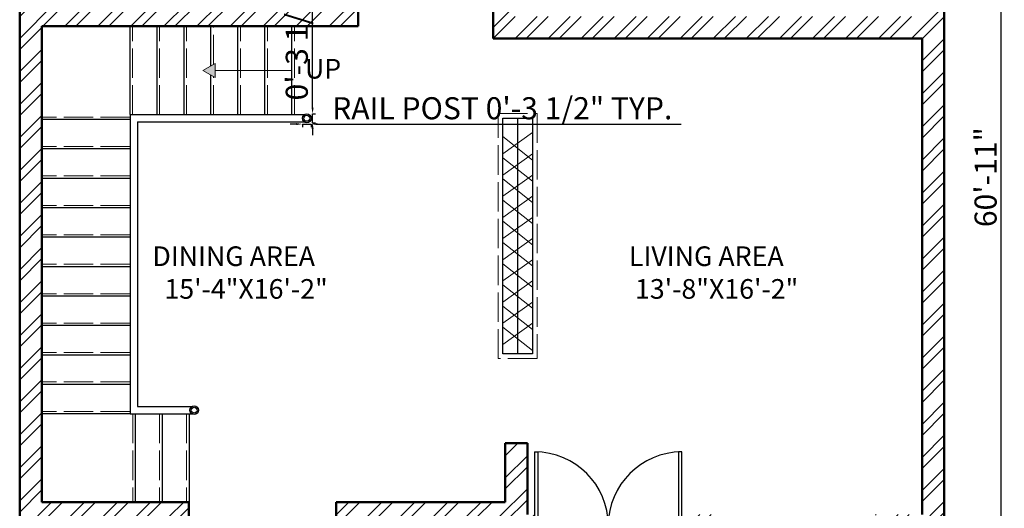
# Model space of a CAD drawing. Units: inches. Extents: x 764 to 1199, y 2696 to 3678.
# Tile 2 of 3: x 777 to 1179, y 3051 to 3250. Entities that reach past the tile are written whole.
import ezdxf

# ---------------------------------------------------------------- set-up
doc = ezdxf.new("R2010")
doc.units = ezdxf.units.IN
doc.linetypes.add('ACAD_ISO02W100', pattern=[15, 12, -3])
for name, color, linetype, lineweight in [('A-ANNO-DIMS', 2, 'Continuous', 18), ('A-ANNO-SYMB', 7, 'Continuous', 18), ('A-ANNO-TEXT', 7, 'Continuous', 18), ('A-AREA-IDEN', 7, 'Continuous', 18), ('A-DOOR', 4, 'Continuous', 25), ('A-FLOR-STRS', 7, 'Continuous', 25), ('A-MILL', 8, 'Continuous', 25), ('A-MILL-HIDN', 8, 'ACAD_ISO02W100', 13), ('A-MILL-PATT', 8, 'Continuous', 13), ('A-STRS-HIDN', 8, 'ACAD_ISO02W100', 13), ('A-WALL', 7, 'Continuous', 50), ('A-WALL-PATT', 252, 'Continuous', 13)]:
    doc.layers.add(name, color=color, linetype=linetype, lineweight=lineweight)
doc.styles.get("Standard").update_dxf_attribs({"font": 'arial.ttf'})
doc.dimstyles.new('ISO-25', dxfattribs={"dimtxt": 9, "dimasz": 2.5, "dimexe": 1.25, "dimexo": 0.625, "dimtad": 1, "dimlunit": 3, "dimtxsty": 'Standard', "dimcen": 2.5, "dimadec": 0, "dimazin": 0, "dimtfac": 1, "dimtmove": 0, "dimatfit": 3, "dimfxl": 1, "dimarcsym": 0})

# ---------------------------------------------------------------- blocks, each defined once
blk = doc.blocks.new('*U2')
for p, q in [((0, 0), (0, -6)), ((40, 0), (40, -6))]:
    blk.add_line(p, q)
blk.add_lwpolyline([(0, 0), (0, 40), (1.75, 40), (1.75, 0)], close=True)
blk.add_arc((0, 0), 40, 0, 90)
blk = doc.blocks.new('*U6')
for p, q in [((0, 0), (0, -6)), ((-40, 0), (-40, -6))]:
    blk.add_line(p, q)
blk.add_lwpolyline([(0, 0), (0, 40), (-1.75, 40), (-1.75, 0)], close=True)
blk.add_arc((0, 0), 40, 90, 180)
blk = doc.blocks.new('*D15')
at = {"layer": 'A-ANNO-DIMS', "color": 0, "lineweight": -2, "transparency": 16777216}
for p, q in [((1154.86, 3551.25), (1178.72, 3551.25)), ((1177.47, 2822.75), (1177.47, 3548.75)), ((1154.86, 2820.25), (1178.72, 2820.25))]:
    blk.add_line(p, q, dxfattribs=at)
at = {"layer": 'A-ANNO-DIMS', "color": 0, "transparency": 16777216}
for points in [[(1177.05, 3548.75), (1177.89, 3548.75), (1177.47, 3551.25)], [(1177.05, 2822.75), (1177.89, 2822.75), (1177.47, 2820.25)]]:
    blk.add_solid(points, dxfattribs=at)
at = {"layer": 'Defpoints', "color": 0, "transparency": 16777216}
for p in [(1154.24, 3551.25), (1177.47, 3551.25), (1154.24, 2820.25)]:
    blk.add_point(p, dxfattribs=at)
at = {"layer": 'A-ANNO-DIMS', "color": 0, "transparency": 16777216, "insert": (1172.25, 3185.75), "char_height": 9, "attachment_point": 5, "rotation": 90}
blk.add_mtext('60\'-11"', dxfattribs=at)
blk = doc.blocks.new('STAIR-RAIL-POST')
for radius in [1.81, 1.21]:
    blk.add_circle((1.81, 1.81), radius)
blk = doc.blocks.new('*D34')
at = {"layer": 'A-ANNO-DIMS', "color": 0, "lineweight": -2, "transparency": 16777216}
for p, q in [((890, 3207.4), (887.5, 3207.4)), ((892.5, 3207.4), (896.12, 3207.4)), ((892.5, 3207.32), (892.5, 3206.15)), ((896.12, 3207.32), (896.12, 3206.15)), ((898.62, 3207.4), (1046.9, 3207.4))]:
    blk.add_line(p, q, dxfattribs=at)
at = {"layer": 'A-ANNO-DIMS', "color": 0, "transparency": 16777216}
for points in [[(890, 3207.82), (890, 3206.98), (892.5, 3207.4)], [(898.62, 3207.82), (898.62, 3206.98), (896.12, 3207.4)]]:
    blk.add_solid(points, dxfattribs=at)
at = {"layer": 'Defpoints', "color": 0, "transparency": 16777216}
for p in [(892.5, 3207.94), (896.12, 3207.94), (896.12, 3207.4)]:
    blk.add_point(p, dxfattribs=at)
at = {"layer": 'A-ANNO-DIMS', "color": 0, "transparency": 16777216, "insert": (974.01, 3212.68), "char_height": 9, "attachment_point": 5}
blk.add_mtext('RAIL POST 0\'-3 1/2" TYP.', dxfattribs=at)
blk = doc.blocks.new('*D35')
at = {"layer": 'A-ANNO-DIMS', "color": 0, "lineweight": -2, "transparency": 16777216}
for p, q in [((896.66, 3214.06), (896.66, 3293.64)), ((896.66, 3207.94), (896.66, 3211.56)), ((896.74, 3211.56), (897.91, 3211.56)), ((896.74, 3207.94), (897.91, 3207.94)), ((896.66, 3205.44), (896.66, 3202.94))]:
    blk.add_line(p, q, dxfattribs=at)
at = {"layer": 'A-ANNO-DIMS', "color": 0, "transparency": 16777216}
for points in [[(896.24, 3214.06), (897.08, 3214.06), (896.66, 3211.56)], [(896.24, 3205.44), (897.08, 3205.44), (896.66, 3207.94)]]:
    blk.add_solid(points, dxfattribs=at)
at = {"layer": 'Defpoints', "color": 0, "transparency": 16777216}
for p in [(896.12, 3211.56), (896.12, 3207.94), (896.66, 3211.56)]:
    blk.add_point(p, dxfattribs=at)
at = {"layer": 'A-ANNO-DIMS', "color": 0, "transparency": 16777216, "insert": (891.38, 3255.1), "char_height": 9, "attachment_point": 5, "rotation": 90}
blk.add_mtext('0\'-3 1/2" TYP.', dxfattribs=at)

msp = doc.modelspace()

# ---------------------------------------------------------------- hatches: boundary and pattern name
at = {"layer": 'A-ANNO-SYMB'}
h = msp.add_hatch(color=256, dxfattribs=at)
h.dxf.hatch_style = 1
h.paths.add_polyline_path([(899.841, 2758.077), (890.705, 2740.978), (909.212, 2740.978)])
h.paths.add_polyline_path([(1023.879, 3009.352), (1018.595, 3000.2), (1029.163, 3000.2)])
h.paths.add_polyline_path([(856.904, 3232.138), (851.903, 3229.25), (856.904, 3226.363)])
at = {"layer": 'A-MILL-PATT'}
h = msp.add_hatch(dxfattribs=at)
h.set_pattern_fill('ANSI31', color=256, scale=2.125626, angle=96.43469, style=0)
h.paths.add_polyline_path([(974.295, 3123.455), (986.295, 3113.887), (986.295, 3200.201), (974.295, 3209.769)])
h = msp.add_hatch(dxfattribs=at)
h.set_pattern_fill('ANSI31', color=256, scale=2.206945, angle=-9.273217, style=0)
h.paths.add_polyline_path([(974.295, 3114.824), (986.295, 3123.455), (986.295, 3209.769), (974.295, 3201.137)])
at = {"layer": 'A-WALL-PATT'}
h = msp.add_hatch(dxfattribs=at)
h.set_pattern_fill('ANSI32', color=256)
h.paths.add_polyline_path([(975.237, 2999.25), (960.237, 2999.25), (960.237, 2993.25), (975.237, 2993.25), (975.237, 2966.771), (984.237, 2966.771), (984.237, 3039.25), (987.237, 3039.25), (987.237, 3043.75), (987.237, 3048.25), (984.237, 3048.25), (984.237, 3053.25), (984.237, 3077.25), (975.237, 3077.25), (975.237, 3053.25), (915.237, 3053.25), (906.237, 3053.25), (906.237, 3047.25), (906.237, 2990.25), (910.737, 2990.25), (915.237, 2990.25), (915.237, 2993.25), (930.237, 2993.25), (930.237, 2999.25), (915.237, 2999.25), (915.237, 3047.25), (975.237, 3047.25)])
h.paths.add_polyline_path([(1047.237, 3048.25), (1047.237, 3043.75), (1047.237, 3039.25), (1066.237, 3039.25), (1066.237, 3048.25)])
h.paths.add_polyline_path([(906.237, 2899.25), (876.237, 2899.25), (876.237, 2890.25), (984.237, 2890.25), (984.237, 2945.771), (975.237, 2945.771), (975.237, 2899.25), (915.237, 2899.25), (915.237, 2960.25), (906.237, 2960.25)])
h.paths.add_polyline_path([(786.237, 3047.25), (846.237, 3047.25), (846.237, 3053.25), (786.237, 3053.25), (786.237, 3247.25), (915.237, 3247.25), (915.237, 3259.25), (906.237, 3259.25), (906.237, 3256.25), (839.237, 3256.25), (839.237, 3271.75), (830.237, 3271.75), (830.237, 3256.25), (786.237, 3256.25), (786.237, 3308.25), (830.237, 3308.25), (830.237, 3292.75), (839.237, 3292.75), (839.237, 3308.25), (906.237, 3308.25), (906.237, 3289.25), (915.237, 3289.25), (915.237, 3320.25), (906.237, 3320.25), (906.237, 3317.25), (786.237, 3317.25), (786.237, 3336.75), (777.237, 3336.75), (777.237, 2890.25), (816.237, 2890.25), (816.237, 2899.25), (786.237, 2899.25)])
h.paths.add_polyline_path([(979.237, 3443.25), (997.737, 3443.25), (997.737, 3452.25), (979.237, 3452.25), (979.237, 3455.25), (970.237, 3455.25), (970.237, 3386.25), (967.237, 3386.25), (967.237, 3377.25), (970.237, 3377.25), (970.237, 3290.25), (979.237, 3290.25)])
h.paths.add_polyline_path([(777.237, 3357.75), (786.237, 3357.75), (786.237, 3377.25), (906.237, 3377.25), (906.237, 3350.25), (915.237, 3350.25), (915.237, 3377.25), (931.237, 3377.25), (931.237, 3386.25), (786.237, 3386.25), (786.237, 3542.25), (970.237, 3542.25), (970.237, 3485.25), (979.237, 3485.25), (979.237, 3542.25), (979.237, 3551.25), (777.237, 3551.25)])
h.paths.add_polyline_path([(1076.237, 3452.25), (1057.737, 3452.25), (1057.737, 3443.25), (1076.237, 3443.25), (1088.237, 3443.25), (1088.237, 3452.25), (1085.237, 3452.25), (1085.237, 3517.523), (1076.237, 3517.523)])
h.paths.add_polyline_path([(913.697, 2904.723), (949.086, 2904.723), (949.086, 2931.714), (913.697, 2931.714)], flags=24)
h = msp.add_hatch(dxfattribs=at)
h.set_pattern_fill('ANSI32', color=256)
h.paths.add_polyline_path([(1154.237, 3551.25), (1076.237, 3551.25), (1076.237, 3542.25), (1076.237, 3538.523), (1085.237, 3538.523), (1085.237, 3542.25), (1145.237, 3542.25), (1145.237, 3452.25), (1118.237, 3452.25), (1118.237, 3443.25), (1145.237, 3443.25), (1145.237, 3251.25), (979.237, 3251.25), (979.237, 3254.25), (970.237, 3254.25), (970.237, 3242.25), (1145.237, 3242.25), (1145.237, 3048.25), (1126.237, 3048.25), (1126.237, 3039.25), (1154.237, 3039.25)])

# ---------------------------------------------------------------- linework, layer by layer
at = {"layer": 'A-ANNO-SYMB'}
msp.add_line((888.237, 3229.25), (856.904, 3229.25), dxfattribs=at)
msp.add_lwpolyline([(851.903, 3229.25), (856.904, 3226.363), (856.904, 3232.138)], close=True, dxfattribs=at)
at = {"layer": 'A-FLOR-STRS'}
for p, q in [((822.237, 3211.25), (822.237, 3247.25)), ((833.237, 3211.25), (833.237, 3247.25)), ((844.237, 3211.25), (844.237, 3247.25)), ((855.237, 3231.175), (855.237, 3247.25)), ((866.237, 3211.25), (866.237, 3247.25)), ((877.237, 3211.25), (877.237, 3247.25)), ((888.237, 3211.25), (888.237, 3247.25)), ((855.237, 3211.25), (855.237, 3227.326)), ((822.237, 3209.25), (786.237, 3209.25)), ((822.237, 3211.25), (893.299, 3211.25)), ((822.237, 3211.25), (822.237, 3089.25)), ((825.237, 3208.25), (893.299, 3208.25)), ((825.237, 3208.25), (825.237, 3092.25)), ((822.237, 3197.25), (786.237, 3197.25)), ((822.237, 3185.25), (786.237, 3185.25)), ((822.237, 3173.25), (786.237, 3173.25)), ((822.237, 3161.25), (786.237, 3161.25)), ((822.237, 3149.25), (786.237, 3149.25)), ((822.237, 3137.25), (786.237, 3137.25)), ((822.237, 3125.25), (786.237, 3125.25)), ((822.237, 3113.25), (786.237, 3113.25)), ((822.237, 3101.25), (786.237, 3101.25)), ((825.237, 3092.25), (847.368, 3092.25)), ((822.237, 3089.25), (786.237, 3089.25)), ((822.237, 3089.25), (847.368, 3089.25)), ((824.309, 3089.25), (824.309, 3053.25)), ((835.309, 3089.25), (835.309, 3053.25)), ((846.309, 3089.25), (846.309, 3053.25))]:
    msp.add_line(p, q, dxfattribs=at)
at = {"layer": 'A-MILL'}
msp.add_line((980.295, 3113.769), (980.295, 3209.769), dxfattribs=at)
msp.add_lwpolyline([(974.295, 3209.769), (986.295, 3209.769), (986.295, 3113.769), (974.295, 3113.769)], close=True, dxfattribs=at)
at = {"layer": 'A-MILL-HIDN'}
msp.add_lwpolyline([(972.295, 3211.769), (988.295, 3211.769), (988.295, 3111.769), (972.295, 3111.769)], close=True, dxfattribs=at)
at = {"layer": 'A-STRS-HIDN'}
for p, q in [((823.237, 3211.25), (823.237, 3247.25)), ((834.237, 3211.25), (834.237, 3247.25)), ((845.237, 3211.25), (845.237, 3247.25)), ((856.237, 3231.753), (856.237, 3247.25)), ((867.237, 3211.25), (867.237, 3247.25)), ((878.237, 3211.25), (878.237, 3247.25)), ((889.237, 3211.25), (889.237, 3247.25)), ((856.237, 3211.25), (856.237, 3226.748)), ((822.237, 3210.25), (786.237, 3210.25)), ((822.237, 3198.25), (786.237, 3198.25)), ((822.237, 3186.25), (786.237, 3186.25)), ((822.237, 3174.25), (786.237, 3174.25)), ((822.237, 3162.25), (786.237, 3162.25)), ((822.237, 3150.25), (786.237, 3150.25)), ((822.237, 3138.25), (786.237, 3138.25)), ((822.237, 3126.25), (786.237, 3126.25)), ((822.237, 3114.25), (786.237, 3114.25)), ((822.237, 3102.25), (786.237, 3102.25)), ((822.237, 3090.25), (786.237, 3090.25)), ((823.309, 3089.25), (823.309, 3053.25)), ((834.309, 3089.25), (834.309, 3053.25)), ((845.309, 3089.25), (845.309, 3053.25))]:
    msp.add_line(p, q, dxfattribs=at)
at = {"layer": 'A-WALL'}
for p, q in [((777.237, 3551.25), (777.237, 2820.25)), ((1154.237, 3551.25), (1154.237, 2820.25)), ((915.237, 3259.25), (915.237, 3247.25)), ((970.237, 3254.25), (970.237, 3242.25)), ((786.237, 3247.25), (915.237, 3247.25)), ((786.237, 3247.25), (786.237, 3053.25)), ((970.237, 3242.25), (1145.237, 3242.25)), ((1145.237, 3242.25), (1145.237, 3048.25)), ((984.237, 3077.25), (975.237, 3077.25)), ((975.237, 3077.25), (975.237, 3053.25)), ((984.237, 3053.25), (984.237, 3077.25)), ((786.237, 3053.25), (846.237, 3053.25)), ((846.237, 3047.25), (846.237, 3053.25)), ((906.237, 3047.25), (906.237, 3053.25)), ((906.237, 3053.25), (915.237, 3053.25)), ((915.237, 3053.25), (975.237, 3053.25)), ((984.237, 3053.25), (984.237, 3048.25))]:
    msp.add_line(p, q, dxfattribs=at)

# ---------------------------------------------------------------- block references
at = {"layer": 'A-DOOR', "xscale": 0.75, "yscale": 0.75, "zscale": 0.75}
for name, p in [('*U2', (987.237, 3043.75)), ('*U6', (1047.237, 3043.75))]:
    msp.add_blockref(name, p, dxfattribs=at)
at = {"layer": 'A-FLOR-STRS'}
for p in [(892.5, 3207.942), (846.569, 3088.942)]:
    msp.add_blockref('STAIR-RAIL-POST', p, dxfattribs=at)

# ---------------------------------------------------------------- texts
at = {"layer": 'A-ANNO-TEXT', "insert": (893.544, 3233.954), "char_height": 8, "attachment_point": 1}
msp.add_mtext_dynamic_manual_height_columns('UP', width=15.69326, gutter_width=12.5, heights=[0], dxfattribs=at)
at = {"layer": 'A-AREA-IDEN', "char_height": 8, "attachment_point": 1}
for s, width, insert in [('DINING AREA\\P  15\'-4"X16\'-2"', 73.10337, (831.367, 3157.529)), ('LIVING AREA\\P 13\'-8"X16\'-2"', 71.36203, (1025.683, 3157.529))]:
    msp.add_mtext_dynamic_manual_height_columns(s, width=width, gutter_width=12.5, heights=[0], dxfattribs=dict(at, insert=insert))

# ---------------------------------------------------------------- dimensions: what is measured, and where the dimension line sits
at = {"layer": 'A-ANNO-DIMS'}
dim = msp.add_linear_dim(base=(1177.47, 3551.25), p1=(1154.237, 2820.25), p2=(1154.237, 3551.25), angle=90, dimstyle='ISO-25', override={"dimclrd": 0, "dimclre": 0, "dimclrt": 0}, dxfattribs=at)
dim.commit()
dim.dimension.update_dxf_attribs({"geometry": '*D15', "text_midpoint": (1172.25, 3185.75)})
dim = msp.add_linear_dim(base=(896.659, 3211.559), p1=(896.117, 3207.942), p2=(896.117, 3211.559), angle=90, text='<> TYP.', dimstyle='ISO-25', override={"dimdec": 1, "dimlfac": 1, "dimrnd": 0, "dimzin": 1, "dimdsep": 46, "dimlunit": 4, "dimfrac": 2}, dxfattribs=at)
dim.commit()
dim.dimension.update_dxf_attribs({"geometry": '*D35', "text_midpoint": (891.378, 3255.099)})
dim = msp.add_linear_dim(base=(896.117, 3207.4), p1=(892.5, 3207.942), p2=(896.117, 3207.942), text='RAIL POST <> TYP.', dimstyle='ISO-25', override={"dimdec": 1, "dimlfac": 1, "dimrnd": 0, "dimzin": 1, "dimdsep": 46, "dimlunit": 4, "dimfrac": 2}, dxfattribs=at)
dim.commit()
dim.dimension.update_dxf_attribs({"geometry": '*D34', "text_midpoint": (974.009, 3212.685)})

doc.saveas('drawing.dxf')
